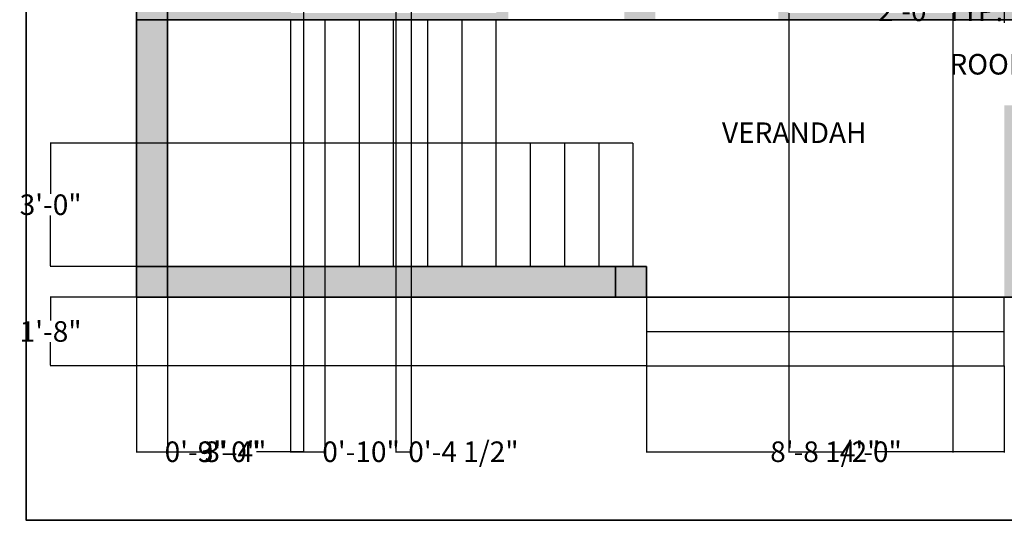
# Model space of a CAD drawing. Units: inches. Extents: x 74 to 548, y 68 to 649.
# Tile 1 of 6: x 81 to 368, y 68 to 214. Entities that reach past the tile are written whole.
import ezdxf

# ---------------------------------------------------------------- set-up
doc = ezdxf.new("R2010")
doc.units = ezdxf.units.IN
doc.header["$MEASUREMENT"] = 0
for name, color, linetype, lineweight in [('A-ANNO-DIMS', 2, 'Continuous', 18), ('A-ANNO-TTLB', 7, 'Continuous', 35), ('A-AREA-IDEN', 7, 'Continuous', 25), ('A-COLS', 7, 'Continuous', 35), ('A-FLOR-STRS', 7, 'Continuous', 25), ('A-WALL', 7, 'Continuous', 35)]:
    doc.layers.add(name, color=color, linetype=linetype, lineweight=lineweight)
doc.layers.add('A-COLS-PATT', color=11, linetype='Continuous', lineweight=13, true_color=0xf27172)
doc.layers.add('A-WALL-PATT', color=7, linetype='Continuous', lineweight=13, true_color=0xffffff)
doc.styles.get("Standard").update_dxf_attribs({"font": 'arial.ttf'})
doc.dimstyles.get("Standard").update_dxf_attribs({"dimtxt": 6, "dimasz": 0.18, "dimexe": 0.18, "dimexo": 0.0625, "dimgap": 0.09, "dimtad": 0, "dimtih": 1, "dimtoh": 1, "dimdec": 1, "dimzin": 0, "dimdsep": 46, "dimlunit": 3, "dimtxsty": 'Standard', "dimcen": 0.09, "dimadec": 0, "dimazin": 0, "dimtfac": 1, "dimtdec": 1, "dimtofl": 0, "dimtmove": 0, "dimatfit": 3, "dimfxl": 1, "dimtolj": 1, "dimtzin": 0, "dimarcsym": 0})

# ---------------------------------------------------------------- blocks, each defined once
blk = doc.blocks.new('*D16')
at = {"layer": 'A-ANNO-DIMS', "color": 0, "lineweight": -2, "transparency": 16777216}
for p, q in [((392.52, 213.24), (396.24, 213.24)), ((396.06, 213.06), (396.06, 204.44)), ((396.06, 189.42), (396.06, 198.05)), ((392.52, 189.24), (396.24, 189.24))]:
    blk.add_line(p, q, dxfattribs=at)
at = {"layer": 'A-ANNO-DIMS', "color": 0, "transparency": 16777216}
for points in [[(396.03, 213.06), (396.09, 213.06), (396.06, 213.24)], [(396.03, 189.42), (396.09, 189.42), (396.06, 189.24)]]:
    blk.add_solid(points, dxfattribs=at)
at = {"layer": 'Defpoints', "color": 0, "transparency": 16777216}
for p in [(392.46, 213.24), (396.06, 213.24), (392.46, 189.24)]:
    blk.add_point(p, dxfattribs=at)
at = {"layer": 'A-ANNO-DIMS', "color": 0, "transparency": 16777216, "insert": (396.06, 201.24), "char_height": 6, "attachment_point": 5}
blk.add_mtext('\\A1;ROOM DOOR 2\'-0" TYP.', dxfattribs=at)
blk = doc.blocks.new('*D17')
at = {"layer": 'A-ANNO-DIMS', "color": 0, "lineweight": -2, "transparency": 16777216}
for p, q in [((368.46, 216.84), (368.28, 216.84)), ((368.46, 213.31), (368.46, 217.02)), ((392.28, 216.84), (368.64, 216.84)), ((392.46, 213.31), (392.46, 217.02))]:
    blk.add_line(p, q, dxfattribs=at)
at = {"layer": 'A-ANNO-DIMS', "color": 0, "transparency": 16777216}
for points in [[(368.64, 216.87), (368.64, 216.81), (368.46, 216.84)], [(392.28, 216.87), (392.28, 216.81), (392.46, 216.84)]]:
    blk.add_solid(points, dxfattribs=at)
at = {"layer": 'Defpoints', "color": 0, "transparency": 16777216}
for p in [(368.46, 216.84), (368.46, 213.24), (392.46, 213.24)]:
    blk.add_point(p, dxfattribs=at)
at = {"layer": 'A-ANNO-DIMS', "color": 0, "transparency": 16777216, "insert": (349.85, 216.84), "char_height": 6, "attachment_point": 5}
blk.add_mtext('\\A1;2\'-0" TYP.', dxfattribs=at)
blk = doc.blocks.new('*D28')
at = {"layer": 'A-ANNO-DIMS', "color": 0, "lineweight": -2, "transparency": 16777216}
for p, q in [((263.82, 133.24), (89.68, 133.24)), ((89.86, 133.06), (89.86, 126.4)), ((89.86, 113.42), (89.86, 120.09)), ((263.82, 113.24), (89.68, 113.24))]:
    blk.add_line(p, q, dxfattribs=at)
at = {"layer": 'A-ANNO-DIMS', "color": 0, "transparency": 16777216}
for points in [[(89.83, 133.06), (89.89, 133.06), (89.86, 133.24)], [(89.83, 113.42), (89.89, 113.42), (89.86, 113.24)]]:
    blk.add_solid(points, dxfattribs=at)
at = {"layer": 'Defpoints', "color": 0, "transparency": 16777216}
for p in [(89.86, 133.24), (263.89, 133.24), (263.89, 113.24)]:
    blk.add_point(p, dxfattribs=at)
at = {"layer": 'A-ANNO-DIMS', "color": 0, "transparency": 16777216, "insert": (89.86, 123.24), "char_height": 6, "attachment_point": 5}
blk.add_mtext('\\A1;1\'-8"', dxfattribs=at)
blk = doc.blocks.new('*D29')
at = {"layer": 'A-ANNO-DIMS', "color": 0, "lineweight": -2, "transparency": 16777216}
for p, q in [((263.89, 113.18), (263.89, 87.96)), ((368.44, 113.18), (368.44, 87.96)), ((264.07, 88.14), (301.11, 88.14)), ((368.26, 88.14), (331.22, 88.14))]:
    blk.add_line(p, q, dxfattribs=at)
at = {"layer": 'A-ANNO-DIMS', "color": 0, "transparency": 16777216}
for points in [[(264.07, 88.17), (264.07, 88.11), (263.89, 88.14)], [(368.26, 88.17), (368.26, 88.11), (368.44, 88.14)]]:
    blk.add_solid(points, dxfattribs=at)
at = {"layer": 'Defpoints', "color": 0, "transparency": 16777216}
for p in [(263.89, 113.24), (368.44, 113.24), (368.44, 88.14)]:
    blk.add_point(p, dxfattribs=at)
at = {"layer": 'A-ANNO-DIMS', "color": 0, "transparency": 16777216, "insert": (316.17, 88.14), "char_height": 6, "attachment_point": 5}
blk.add_mtext('\\A1;8\'-8 1/2"', dxfattribs=at)
blk = doc.blocks.new('*D31')
at = {"layer": 'A-ANNO-DIMS', "color": 0, "lineweight": -2, "transparency": 16777216}
for p, q in [((305.46, 216.18), (305.46, 87.96)), ((353.46, 216.18), (353.46, 87.96)), ((305.64, 88.14), (321.28, 88.14)), ((353.28, 88.14), (337.65, 88.14))]:
    blk.add_line(p, q, dxfattribs=at)
at = {"layer": 'A-ANNO-DIMS', "color": 0, "transparency": 16777216}
for points in [[(305.64, 88.17), (305.64, 88.11), (305.46, 88.14)], [(353.28, 88.17), (353.28, 88.11), (353.46, 88.14)]]:
    blk.add_solid(points, dxfattribs=at)
at = {"layer": 'Defpoints', "color": 0, "transparency": 16777216}
for p in [(305.46, 216.24), (353.46, 216.24), (353.46, 88.14)]:
    blk.add_point(p, dxfattribs=at)
at = {"layer": 'A-ANNO-DIMS', "color": 0, "transparency": 16777216, "insert": (329.46, 88.14), "char_height": 6, "attachment_point": 5}
blk.add_mtext('\\A1;4\'-0"', dxfattribs=at)
blk = doc.blocks.new('*D32')
at = {"layer": 'A-ANNO-DIMS', "color": 0, "lineweight": -2, "transparency": 16777216}
for p, q in [((159.9, 178.24), (89.68, 178.24)), ((89.86, 178.06), (89.86, 163.4)), ((89.86, 142.42), (89.86, 157.09)), ((159.9, 142.24), (89.68, 142.24))]:
    blk.add_line(p, q, dxfattribs=at)
at = {"layer": 'A-ANNO-DIMS', "color": 0, "transparency": 16777216}
for points in [[(89.83, 178.06), (89.89, 178.06), (89.86, 178.24)], [(89.83, 142.42), (89.89, 142.42), (89.86, 142.24)]]:
    blk.add_solid(points, dxfattribs=at)
at = {"layer": 'Defpoints', "color": 0, "transparency": 16777216}
for p in [(89.86, 178.24), (159.96, 178.24), (159.96, 142.24)]:
    blk.add_point(p, dxfattribs=at)
at = {"layer": 'A-ANNO-DIMS', "color": 0, "transparency": 16777216, "insert": (89.86, 160.24), "char_height": 6, "attachment_point": 5}
blk.add_mtext('\\A1;3\'-0"', dxfattribs=at)
blk = doc.blocks.new('*D33')
at = {"layer": 'A-ANNO-DIMS', "color": 0, "lineweight": -2, "transparency": 16777216}
for p, q in [((159.96, 142.18), (159.96, 87.96)), ((169.96, 142.18), (169.96, 87.96)), ((160.14, 88.14), (169.78, 88.14)), ((169.96, 88.14), (170.14, 88.14))]:
    blk.add_line(p, q, dxfattribs=at)
at = {"layer": 'A-ANNO-DIMS', "color": 0, "transparency": 16777216}
for points in [[(160.14, 88.17), (160.14, 88.11), (159.96, 88.14)], [(169.78, 88.17), (169.78, 88.11), (169.96, 88.14)]]:
    blk.add_solid(points, dxfattribs=at)
at = {"layer": 'Defpoints', "color": 0, "transparency": 16777216}
for p in [(159.96, 142.24), (169.96, 142.24), (169.96, 88.14)]:
    blk.add_point(p, dxfattribs=at)
at = {"layer": 'A-ANNO-DIMS', "color": 0, "transparency": 16777216, "insert": (180.54, 88.14), "char_height": 6, "attachment_point": 5}
blk.add_mtext('\\A1;0\'-10"', dxfattribs=at)
blk = doc.blocks.new('*D34')
at = {"layer": 'A-ANNO-DIMS', "color": 0, "lineweight": -2, "transparency": 16777216}
for p, q in [((114.96, 133.18), (114.96, 87.96)), ((123.96, 133.18), (123.96, 87.96)), ((115.14, 88.14), (123.78, 88.14)), ((123.96, 88.14), (124.14, 88.14))]:
    blk.add_line(p, q, dxfattribs=at)
at = {"layer": 'A-ANNO-DIMS', "color": 0, "transparency": 16777216}
for points in [[(115.14, 88.17), (115.14, 88.11), (114.96, 88.14)], [(123.78, 88.17), (123.78, 88.11), (123.96, 88.14)]]:
    blk.add_solid(points, dxfattribs=at)
at = {"layer": 'Defpoints', "color": 0, "transparency": 16777216}
for p in [(114.96, 133.24), (123.96, 133.24), (123.96, 88.14)]:
    blk.add_point(p, dxfattribs=at)
at = {"layer": 'A-ANNO-DIMS', "color": 0, "transparency": 16777216, "insert": (132.21, 88.14), "char_height": 6, "attachment_point": 5}
blk.add_mtext('\\A1;0\'-9"', dxfattribs=at)
blk = doc.blocks.new('*D35')
at = {"layer": 'A-ANNO-DIMS', "color": 0, "lineweight": -2, "transparency": 16777216}
for p, q in [((190.71, 365.68), (190.71, 87.96)), ((195.21, 365.68), (195.21, 87.96)), ((190.89, 88.14), (195.03, 88.14)), ((195.21, 88.14), (195.39, 88.14))]:
    blk.add_line(p, q, dxfattribs=at)
at = {"layer": 'A-ANNO-DIMS', "color": 0, "transparency": 16777216}
for points in [[(190.89, 88.17), (190.89, 88.11), (190.71, 88.14)], [(195.03, 88.17), (195.03, 88.11), (195.21, 88.14)]]:
    blk.add_solid(points, dxfattribs=at)
at = {"layer": 'Defpoints', "color": 0, "transparency": 16777216}
for p in [(190.71, 365.74), (195.21, 365.74), (195.21, 88.14)]:
    blk.add_point(p, dxfattribs=at)
at = {"layer": 'A-ANNO-DIMS', "color": 0, "transparency": 16777216, "insert": (210.45, 88.14), "char_height": 6, "attachment_point": 5}
blk.add_mtext('\\A1;0\'-4 1/2"', dxfattribs=at)
blk = doc.blocks.new('*D38')
at = {"layer": 'A-ANNO-DIMS', "color": 0, "lineweight": -2, "transparency": 16777216}
for p, q in [((159.96, 142.18), (159.96, 87.96)), ((123.96, 133.18), (123.96, 87.96)), ((124.14, 88.14), (133.9, 88.14)), ((159.78, 88.14), (150.02, 88.14))]:
    blk.add_line(p, q, dxfattribs=at)
at = {"layer": 'A-ANNO-DIMS', "color": 0, "transparency": 16777216}
for points in [[(124.14, 88.17), (124.14, 88.11), (123.96, 88.14)], [(159.78, 88.17), (159.78, 88.11), (159.96, 88.14)]]:
    blk.add_solid(points, dxfattribs=at)
at = {"layer": 'Defpoints', "color": 0, "transparency": 16777216}
for p in [(159.96, 142.24), (123.96, 133.24), (159.96, 88.14)]:
    blk.add_point(p, dxfattribs=at)
at = {"layer": 'A-ANNO-DIMS', "color": 0, "transparency": 16777216, "insert": (141.96, 88.14), "char_height": 6, "attachment_point": 5}
blk.add_mtext('\\A1;3\'-0"', dxfattribs=at)
blk = doc.blocks.new('*D44')
at = {"layer": 'A-ANNO-DIMS', "color": 0, "lineweight": -2, "transparency": 16777216}
for p, q in [((163.71, 448.18), (163.71, 87.96)), ((123.96, 439.18), (123.96, 87.96)), ((124.14, 88.14), (135.77, 88.14)), ((163.53, 88.14), (151.9, 88.14))]:
    blk.add_line(p, q, dxfattribs=at)
at = {"layer": 'A-ANNO-DIMS', "color": 0, "transparency": 16777216}
for points in [[(124.14, 88.17), (124.14, 88.11), (123.96, 88.14)], [(163.53, 88.17), (163.53, 88.11), (163.71, 88.14)]]:
    blk.add_solid(points, dxfattribs=at)
at = {"layer": 'Defpoints', "color": 0, "transparency": 16777216}
for p in [(163.71, 448.24), (123.96, 439.24), (163.71, 88.14)]:
    blk.add_point(p, dxfattribs=at)
at = {"layer": 'A-ANNO-DIMS', "color": 0, "transparency": 16777216, "insert": (143.84, 88.14), "char_height": 6, "attachment_point": 5}
blk.add_mtext('\\A1;3\'-4"', dxfattribs=at)

msp = doc.modelspace()

# ---------------------------------------------------------------- hatches: boundary and pattern name
at = {"layer": 'A-COLS-PATT'}
h = msp.add_hatch(color=256, dxfattribs=at)
h.dxf.hatch_style = 1
h.paths.add_polyline_path([(123.96, 584.24), (114.96, 584.24), (114.96, 575.24), (123.96, 575.24)])
h.paths.add_polyline_path([(266.46, 584.24), (257.46, 584.24), (257.46, 575.24), (266.46, 575.24)])
h.paths.add_polyline_path([(329.46, 584.24), (320.46, 584.24), (320.46, 575.24), (329.46, 575.24)])
h.paths.add_polyline_path([(471.96, 584.24), (462.96, 584.24), (462.96, 575.24), (471.96, 575.24)])
h.paths.add_polyline_path([(123.96, 448.24), (114.96, 448.24), (114.96, 439.24), (123.96, 439.24)])
h.paths.add_polyline_path([(266.46, 448.24), (261.96, 448.24), (257.46, 448.24), (257.46, 439.24), (266.46, 439.24)])
h.paths.add_polyline_path([(329.46, 448.24), (320.46, 448.24), (320.46, 439.24), (329.46, 439.24)])
h.paths.add_polyline_path([(471.96, 448.24), (462.96, 448.24), (462.96, 439.24), (471.96, 439.24)])
h.paths.add_polyline_path([(123.96, 365.74), (114.96, 365.74), (114.96, 356.74), (123.96, 356.74)])
h.paths.add_polyline_path([(266.46, 365.74), (257.46, 365.74), (257.46, 356.74), (266.46, 356.74)])
h.paths.add_polyline_path([(123.96, 223.24), (114.96, 223.24), (114.96, 214.24), (123.96, 214.24)])
h.paths.add_polyline_path([(266.46, 223.24), (257.46, 223.24), (257.46, 214.24), (266.46, 214.24)])
h.paths.add_polyline_path([(123.96, 142.24), (114.96, 142.24), (114.96, 133.24), (123.96, 133.24)])
h.paths.add_polyline_path([(263.89, 142.24), (254.89, 142.24), (254.89, 133.24), (263.89, 133.24)])
h.paths.add_polyline_path([(471.96, 142.24), (462.96, 142.24), (462.96, 133.24), (471.96, 133.24)])
h.paths.add_polyline_path([(377.46, 142.24), (368.46, 142.24), (368.46, 133.24), (377.46, 133.24)])
h.paths.add_polyline_path([(377.46, 223.24), (368.46, 223.24), (368.46, 214.24), (377.46, 214.24)])
h.paths.add_polyline_path([(471.96, 223.24), (462.96, 223.24), (462.96, 214.24), (471.96, 214.24)])
h.paths.add_polyline_path([(471.96, 298.99), (462.96, 298.99), (462.96, 289.99), (471.96, 289.99)])
h.paths.add_polyline_path([(471.96, 365.74), (462.96, 365.74), (462.96, 356.74), (471.96, 356.74)])
at = {"layer": 'A-WALL-PATT'}
h = msp.add_hatch(color=256, dxfattribs=at)
h.dxf.hatch_style = 1
h.paths.add_polyline_path([(123.96, 356.74), (114.96, 356.74), (114.96, 223.24), (123.96, 223.24)])
h.paths.add_polyline_path([(123.96, 439.24), (114.96, 439.24), (114.96, 365.74), (123.96, 365.74)])
h.paths.add_polyline_path([(123.96, 575.24), (114.96, 575.24), (114.96, 448.24), (123.96, 448.24)])
h.paths.add_polyline_path([(257.46, 584.24), (123.96, 584.24), (123.96, 575.24), (257.46, 575.24)])
h.paths.add_polyline_path([(266.46, 575.24), (261.96, 575.24), (261.96, 490.24), (266.46, 490.24)])
h.paths.add_polyline_path([(266.46, 454.24), (261.96, 454.24), (261.96, 448.24), (266.46, 448.24)])
h.paths.add_polyline_path([(257.46, 448.24), (187.71, 448.24), (187.71, 443.74), (190.71, 443.74), (190.71, 365.74), (123.96, 365.74), (123.96, 361.24), (257.46, 361.24), (257.46, 365.74), (195.21, 365.74), (195.21, 443.74), (257.46, 443.74)])
h.paths.add_polyline_path([(163.71, 448.24), (123.96, 448.24), (123.96, 443.74), (163.71, 443.74)], flags=17)
h.paths.add_polyline_path([(223.59, 223.24), (220.05, 223.24), (220.05, 216.24), (160.05, 216.24), (160.05, 223.24), (123.96, 223.24), (123.96, 214.24), (159.96, 214.24), (223.59, 214.24)])
h.paths.add_polyline_path([(123.96, 214.24), (114.96, 214.24), (114.96, 142.24), (123.96, 142.24)])
h.paths.add_polyline_path([(254.89, 142.24), (123.96, 142.24), (123.96, 133.24), (254.89, 133.24)])
h.paths.add_polyline_path([(462.96, 142.24), (377.46, 142.24), (377.46, 133.24), (462.96, 133.24)])
h.paths.add_polyline_path([(372.96, 189.24), (368.46, 189.24), (368.46, 142.24), (372.96, 142.24)])
h.paths.add_polyline_path([(471.96, 214.24), (462.96, 214.24), (462.96, 142.24), (471.96, 142.24)])
h.paths.add_polyline_path([(462.96, 223.24), (403.93, 223.24), (403.93, 294.49), (409.93, 294.49), (409.93, 298.99), (403.93, 298.99), (399.43, 298.99), (399.43, 223.24), (377.46, 223.24), (377.46, 214.24), (462.96, 214.24)])
h.paths.add_polyline_path([(368.46, 223.24), (353.46, 223.24), (353.46, 216.24), (305.46, 216.24), (305.46, 223.24), (302.46, 223.24), (302.46, 214.24), (368.46, 214.24)])
h.paths.add_polyline_path([(471.96, 289.99), (462.96, 289.99), (462.96, 223.24), (471.96, 223.24)])
h.paths.add_polyline_path([(462.96, 298.99), (433.93, 298.99), (433.93, 294.49), (462.96, 294.49)], flags=0)
h.paths.add_polyline_path([(471.96, 356.74), (462.96, 356.74), (462.96, 298.99), (471.96, 298.99)])
h.paths.add_polyline_path([(462.96, 365.74), (403.93, 365.74), (403.93, 361.24), (462.96, 361.24)], flags=17)
h.paths.add_polyline_path([(471.96, 439.24), (462.96, 439.24), (462.96, 365.74), (471.96, 365.74)])
h.paths.add_polyline_path([(462.96, 448.24), (329.46, 448.24), (329.46, 439.24), (368.46, 439.24), (368.46, 361.24), (372.96, 361.24), (372.96, 443.74), (462.96, 443.74)])
h.paths.add_polyline_path([(324.96, 454.24), (320.46, 454.24), (320.46, 448.24), (324.96, 448.24)])
h.paths.add_polyline_path([(471.96, 575.24), (462.96, 575.24), (462.96, 448.24), (471.96, 448.24)])
h.paths.add_polyline_path([(462.96, 584.24), (329.46, 584.24), (329.46, 575.24), (462.96, 575.24)])
h.paths.add_polyline_path([(320.46, 584.24), (266.46, 584.24), (266.46, 575.24), (320.46, 575.24)])
h.paths.add_polyline_path([(324.96, 575.24), (320.46, 575.24), (320.46, 490.24), (324.96, 490.24)])
h.paths.add_polyline_path([(266.46, 405.58), (257.46, 405.58), (257.46, 365.74), (266.46, 365.74)])
h.paths.add_polyline_path([(266.46, 356.74), (261.96, 356.74), (261.96, 333.81), (266.46, 333.81)])
h.paths.add_polyline_path([(266.46, 297.81), (261.96, 297.81), (261.96, 223.24), (266.46, 223.24)])

# ---------------------------------------------------------------- linework, layer by layer
at = {"layer": 'A-ANNO-TTLB'}
msp.add_lwpolyline([(82.75, 649.38), (548.44, 649.38), (548.44, 68.13), (82.75, 68.13)], close=True, dxfattribs=at)
at = {"layer": 'A-COLS'}
for p, q in [((254.89, 133.24), (254.89, 142.24)), ((263.89, 142.24), (263.89, 133.24))]:
    msp.add_line(p, q, dxfattribs=at)
at = {"layer": 'A-FLOR-STRS'}
for p, q in [((159.96, 214.24), (159.96, 142.24)), ((169.96, 214.24), (169.96, 142.24)), ((179.96, 214.24), (179.96, 142.24)), ((189.96, 214.24), (189.96, 142.24)), ((199.96, 214.24), (199.96, 142.24)), ((209.96, 214.24), (209.96, 142.24)), ((219.96, 214.24), (219.96, 142.24)), ((259.96, 178.24), (159.96, 178.24)), ((229.96, 178.24), (229.96, 142.24)), ((239.96, 178.24), (239.96, 142.24)), ((249.96, 178.24), (249.96, 142.24)), ((259.96, 178.24), (259.96, 142.24)), ((263.89, 133.24), (263.89, 113.24)), ((368.44, 113.24), (368.44, 133.24)), ((263.89, 123.24), (368.44, 123.24)), ((263.89, 113.24), (368.44, 113.24))]:
    msp.add_line(p, q, dxfattribs=at)
at = {"layer": 'A-WALL'}
for p, q in [((114.96, 584.24), (114.96, 133.24)), ((123.96, 584.24), (123.96, 133.24)), ((114.96, 214.24), (471.96, 214.24)), ((123.96, 214.24), (159.96, 214.24)), ((114.96, 142.24), (263.89, 142.24)), ((114.96, 133.24), (471.96, 133.24))]:
    msp.add_line(p, q, dxfattribs=at)

# ---------------------------------------------------------------- texts
at = {"layer": 'A-AREA-IDEN', "insert": (285.98, 184.26), "char_height": 6, "attachment_point": 1}
msp.add_mtext_dynamic_manual_height_columns('VERANDAH', width=55.2018, gutter_width=30, heights=[0], dxfattribs=at)

# ---------------------------------------------------------------- dimensions: what is measured, and where the dimension line sits
at = {"layer": 'A-ANNO-DIMS'}
for base, p1, p2, picture, middle in [((163.710646, 88.142592), (123.960646, 439.242592), (163.710646, 448.242592), '*D44', (143.835646, 88.142592)), ((195.21, 88.14), (190.71, 365.74), (195.21, 365.74), '*D35', (210.45, 88.14)), ((353.46, 88.14), (305.46, 216.24), (353.46, 216.24), '*D31', (329.46, 88.14)), ((159.96, 88.14), (123.96, 133.24), (159.96, 142.24), '*D38', (141.96, 88.14)), ((169.96, 88.14), (159.96, 142.24), (169.96, 142.24), '*D33', (180.54, 88.14)), ((123.96, 88.14), (114.96, 133.24), (123.96, 133.24), '*D34', (132.21, 88.14)), ((368.443, 88.1426), (263.8873, 113.2426), (368.443, 113.2426), '*D29', (316.1652, 88.1426))]:
    dim = msp.add_linear_dim(base=base, p1=p1, p2=p2, dimstyle='Standard', override={"dimdec": 1, "dimlfac": 1, "dimrnd": 0, "dimzin": 1, "dimdsep": 46, "dimlunit": 4, "dimfrac": 2}, dxfattribs=at)
    dim.commit()
    dim.dimension.update_dxf_attribs({"geometry": picture, "text_midpoint": middle})
for base, p1, p2, angle, text, picture, middle in [((368.46, 216.84), (392.46, 213.24), (368.46, 213.24), 180, '<> TYP.', '*D17', (349.85, 216.84)), ((396.06, 213.24), (392.46, 189.24), (392.46, 213.24), 90, 'ROOM DOOR <> TYP.', '*D16', (396.06, 201.24))]:
    dim = msp.add_linear_dim(base=base, p1=p1, p2=p2, angle=angle, text=text, dimstyle='Standard', override={"dimdec": 1, "dimlfac": 1, "dimrnd": 0, "dimzin": 1, "dimdsep": 46, "dimlunit": 4, "dimfrac": 2}, dxfattribs=at)
    dim.commit()
    dim.dimension.update_dxf_attribs({"geometry": picture, "text_midpoint": middle})
for base, p1, p2, picture, middle in [((89.86, 178.24), (159.96, 142.24), (159.96, 178.24), '*D32', (89.86, 160.24)), ((89.86, 133.24), (263.89, 113.24), (263.89, 133.24), '*D28', (89.86, 123.24))]:
    dim = msp.add_linear_dim(base=base, p1=p1, p2=p2, angle=90, dimstyle='Standard', override={"dimdec": 1, "dimlfac": 1, "dimrnd": 0, "dimzin": 1, "dimdsep": 46, "dimlunit": 4, "dimfrac": 2}, dxfattribs=at)
    dim.commit()
    dim.dimension.update_dxf_attribs({"geometry": picture, "text_midpoint": middle})

doc.saveas('drawing.dxf')
